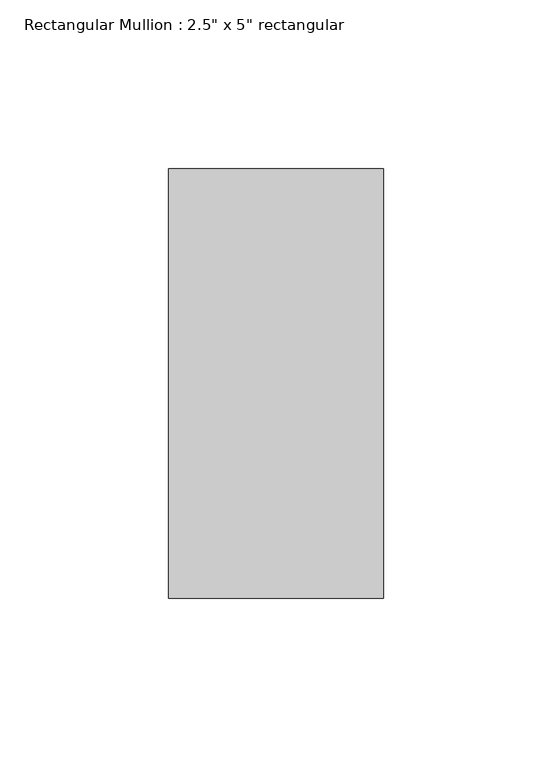
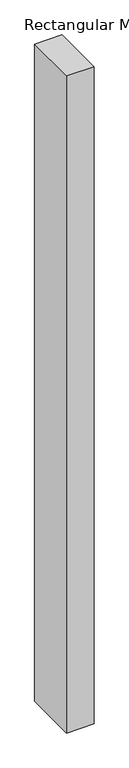
"""IFC4 building model written with IfcOpenShell, lengths in millimetres: member geometry."""

from ifc_helpers import new_model, si_unit, frame, origin, place, context, project, spatial, polyline, outline, extrude, source, transform, mapped, element, save


def member_3f35b8d2(model_context):
    return source(origin(), model_context, "Body", "SweptSolid", [
        extrude(outline(polyline([(0.0, 63.5), (0.0, -63.5), (-63.5, -63.5), (-63.5, 63.5), (0.0, 63.5)])), frame((0.0, 0.0, -1600.1465467), z_axis=(0.0, 0.0, 1.0), x_axis=(1.0, 0.0, 0.0)), (0.0, 0.0, 1.0), 1600.1465467),
    ])


if __name__ == "__main__":
    model = new_model("IFC4")
    model_context = context("Model", 3, world=origin())
    ifc_project = project(units=[si_unit("LENGTHUNIT", "METRE", prefix="MILLI")], contexts=[model_context])
    site = spatial("IfcSite", under=ifc_project)
    building = spatial("IfcBuilding", under=site)
    placement = place(None, origin())
    member_shape = member_3f35b8d2(model_context)
    element("IfcMember", 1, ObjectType="Rectangular Mullion : 2.5\" x 5\" rectangular", at=placement, inside=building, context=model_context, shape_type="MappedRepresentation", body=[
        mapped(member_shape, transform((0.0, 0.0, 0.0), x_axis=(1.0, 0.0, 0.0), y_axis=(0.0, 1.0, 0.0), z_axis=(0.0, 0.0, 1.0))),
    ])
    save(model, "model.ifc")

# Revit data of these elements
# Type "Rectangular Mullion : 2.5\" x 5\" rectangular"
#   built-in parameter 1007304 = 0.416667 (stored number, unit not read)
#   built-in parameter 1007301 = 0.104167 (stored number, unit not read)
#   built-in parameter 1007300 = 0.104167 (stored number, unit not read)
# Element 1 (IfcMember, "Rectangular Mullion : 2.5\" x 5\" rectangular")
#   Materials on its faces: "Aluminum"
# Materials
#   "Aluminum": class "Metal", colour RGB 247 247 247, transparency 0, Description = "Aluminum 6061", Cost = 0
